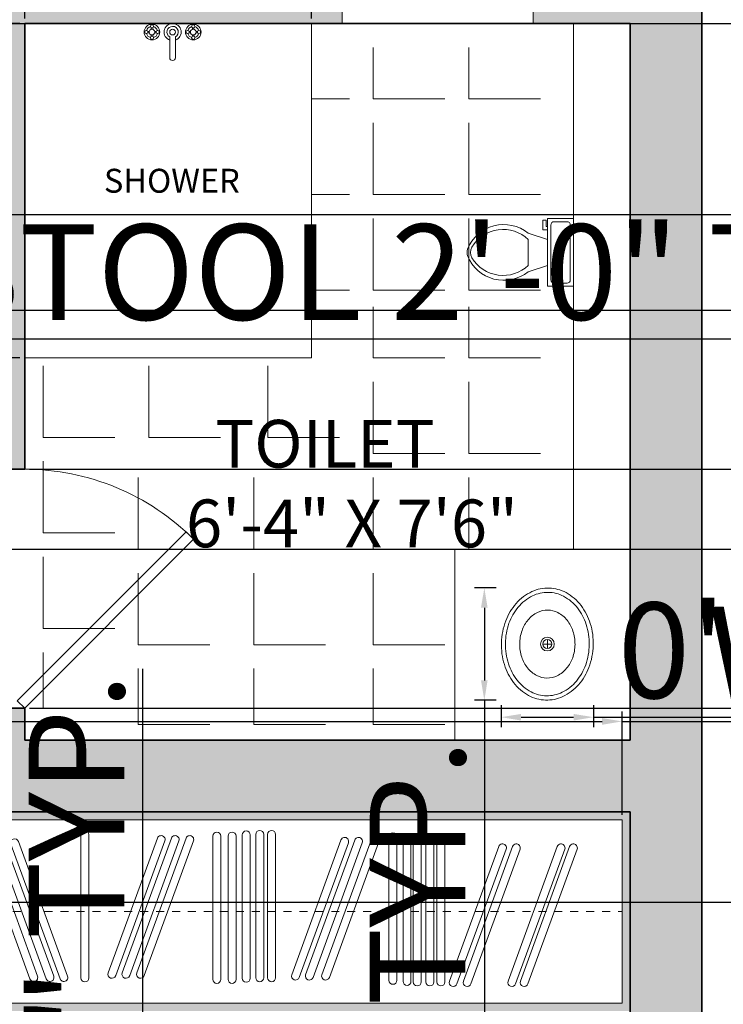
# Model space of a CAD drawing. Units: millimetres. Extents: x 542930 to 543750, y 628093 to 628738.
# Tile 10 of 14: x 543414 to 543502, y 628458 to 628581. Entities that reach past the tile are written whole.
import ezdxf

# ---------------------------------------------------------------- set-up
doc = ezdxf.new("R2010")
doc.units = ezdxf.units.MM
doc.linetypes.add('JIS_02_1.0', pattern=[2, 1, -1])
for name, color, linetype, lineweight in [('A-ANNO-DIMS', 2, 'Continuous', 18), ('A-FLOR-FIXT', 9, 'Continuous', 18), ('A-FURN-MILL', 8, 'Continuous', 18), ('A-FURN-MILL-HIDN', 8, 'JIS_02_1.0', 13), ('A-FURN-PATT', 9, 'Continuous', 13), ('A-WALL', 7, 'Continuous', 35), ('DOORS', 30, 'Continuous', 18), ('WINDOW', 70, 'Continuous', 18)]:
    doc.layers.add(name, color=color, linetype=linetype, lineweight=lineweight)
for name, color, linetype, lineweight, true_color in [('A-ANNO-TEXT', 40, 'Continuous', 18, 0xf8d731), ('A-AREA-IDEN', 40, 'Continuous', 18, 0xf8d731), ('A-FLOR-PATT', 241, 'Continuous', 13, 0xf7abae), ('A-WALL-PATT', 251, 'Continuous', 13, 0x636466)]:
    doc.layers.add(name, color=color, linetype=linetype, lineweight=lineweight, true_color=true_color)
doc.styles.get("Standard").update_dxf_attribs({"font": 'arial.ttf'})
doc.dimstyles.new('ISO-25', dxfattribs={"dimtxt": 12, "dimasz": 2.5, "dimexe": 1.25, "dimexo": 0.625, "dimtad": 1, "dimdec": 0, "dimlunit": 3, "dimtxsty": 'Standard', "dimcen": 2.5, "dimadec": 0, "dimazin": 0, "dimtfac": 1, "dimtdec": 0, "dimtmove": 0, "dimatfit": 3, "dimfxl": 1, "dimarcsym": 0})

# ---------------------------------------------------------------- blocks, each defined once
blk = doc.blocks.new('*U3')
for p, q in [((-40, 0), (-40, -6)), ((0, 0), (0, -6))]:
    blk.add_line(p, q)
blk.add_lwpolyline([(0, 0), (-28.28, 28.28), (-29.52, 27.05), (-1.24, -1.24)], close=True)
blk.add_arc((0, 0), 40, 135, 180)
blk = doc.blocks.new('*U6')
for p, q in [((9.5, -6), (9.5, -2)), ((-10, -8.5), (-8, -8.5)), ((-10, -9.5), (-10, -8.5)), ((-8, -8.5), (-8, -8)), ((-7, -8), (-7, -9.5)), ((-4, -8), (-6, -14)), ((4, -8), (6, -14)), ((-7, -9.5), (-10, -9.5)), ((4, -14), (-4, -14))]:
    blk.add_line(p, q)
blk.add_lwpolyline([(10.5, -8), (10.5, 0), (-10.5, 0), (-10.5, -8)], close=True)
for points in [[(-9.5, -2), (-9.5, -6)], [(8.5, -1), (-8.5, -1)], [(-8.5, -7), (8.5, -7)]]:
    blk.add_lwpolyline(points)
for centre, radius, start, end in [((-8.62, -1.88), 0.884, 81.8699, 188.1301), ((8.62, -1.88), 0.884, 351.8699, 98.1301), ((-8.62, -6.12), 0.884, 171.8699, 278.1301), ((8.62, -6.12), 0.884, 261.8699, 8.1301), ((3.52, -21.58), 12.17, 141.4691, 247.9714), ((4.2, -21.82), 11.33, 136.3677, 238.9468), ((-3.52, -21.58), 12.17, 292.0284, 38.5307), ((-4.2, -21.82), 11.33, 301.053, 43.6321), ((0, -27.88), 4, 245.7318, 294.2682), ((0, -29), 4, 254.8605, 285.1395)]:
    blk.add_arc(centre, radius, start, end)
blk = doc.blocks.new('Sink - Oval top')
for p, q in [((-1, 0), (1, 0)), ((0, 1), (0, -1))]:
    blk.add_line(p, q)
for points in [[(-12.23, 0.39, 0.117634), (-11.46, -3.36, 0.104469), (-8.88, -6.8, 0.090016), (-5.08, -9.07, 0.08192), (-0.32, -10.02, 0.08192), (4.49, -9.38, 0.090016), (8.42, -7.36, 0.104469), (11.22, -4.09, 0.117634), (12.23, -0.39, 0.117634), (11.46, 3.36, 0.104469), (8.88, 6.8, 0.090016), (5.08, 9.07, 0.08192), (0.32, 10.02, 0.08192), (-4.49, 9.38, 0.090016), (-8.42, 7.36, 0.104469), (-11.22, 4.09, 0.117634)], [(-11.29, 0.16, 0.118622), (-10.52, -3.25, 0.104678), (-8.07, -6.36, 0.089562), (-4.54, -8.37, 0.081185), (-0.13, -9.15, 0.081185), (4.3, -8.49, 0.089562), (7.89, -6.58, 0.104678), (10.42, -3.55, 0.118622), (11.29, -0.16, 0.118622), (10.52, 3.25, 0.104678), (8.07, 6.36, 0.089562), (4.54, 8.37, 0.081185), (0.13, 9.15, 0.081185), (-4.3, 8.49, 0.089562), (-7.89, 6.58, 0.104678), (-10.42, 3.55, 0.118622)], [(-7.42, 0.08, 0.118283), (-6.91, -2.17, 0.104607), (-5.29, -4.21, 0.089718), (-2.97, -5.53, 0.081436), (-0.07, -6.04, 0.081436), (2.84, -5.59, 0.089718), (5.2, -4.33, 0.104607), (6.86, -2.32, 0.118283), (7.42, -0.08, 0.118283), (6.91, 2.17, 0.104607), (5.29, 4.21, 0.089718), (2.97, 5.53, 0.081436), (0.07, 6.04, 0.081436), (-2.84, 5.59, 0.089718), (-5.2, 4.33, 0.104607), (-6.86, 2.32, 0.118283)]]:
    blk.add_lwpolyline(points, format="xyb", close=True)
for radius in [1.5, 1]:
    blk.add_circle((0, 0), radius)
blk = doc.blocks.new('Faucet - Bathroom top')
for p, q in [((-4.107, 0.125), (-4.375, 0.125)), ((-3.75, 0.4788), (-3.75, 0.75)), ((-3.5, 0.482), (-3.5, 0.75)), ((-3.1461, 0.125), (-2.875, 0.125)), ((3.143, 0.125), (2.875, 0.125)), ((3.5, 0.4788), (3.5, 0.75)), ((3.75, 0.482), (3.75, 0.75)), ((4.1039, 0.125), (4.375, 0.125)), ((-4.1039, -0.125), (-4.375, -0.125)), ((-3.75, -0.4821), (-3.75, -0.75)), ((-3.5, -0.4789), (-3.5, -0.75)), ((-3.143, -0.125), (-2.875, -0.125)), ((-0.5, -0.8639), (-0.5, -4.5)), ((0.5, -4.5), (0.5, -0.8631)), ((3.1461, -0.125), (2.875, -0.125)), ((3.5, -0.4821), (3.5, -0.75)), ((3.75, -0.4789), (3.75, -0.75)), ((4.107, -0.125), (4.375, -0.125))]:
    blk.add_line(p, q)
for centre, radius in [((-3.625, 0), 1.375), ((-4.625, 0), 0.2795), ((-3.625, 0), 0.5), ((-3.625, 1), 0.2795), ((-2.625, 0), 0.2795), ((0, 0), 0.5), ((3.625, 0), 1.375), ((2.625, 0), 0.2795), ((3.625, 0), 0.5), ((3.625, 1), 0.2795), ((4.625, 0), 0.2795), ((-3.625, -1), 0.2795), ((3.625, -1), 0.2795)]:
    blk.add_circle(centre, radius)
for centre, radius, start, end in [((-3.625, 0), 1, 105.2407, 164.2093), ((-3.625, 0), 1, 16.44125, 74.07887), ((0, 0), 1.5, 289.6514, 250.3603), ((0, 0), 1, 300.3431, 239.7554), ((3.625, 0), 1, 106.12, 164.0884), ((3.625, 0), 1, 16.23422, 73.90469), ((-3.625, 0), 1, 196.2342, 253.9047), ((-3.625, 0), 1, 286.12, 344.0884), ((3.625, 0), 1, 196.4413, 254.0789), ((3.625, 0), 1, 285.2407, 344.2093), ((0, -4.5), 0.5, 180, 0)]:
    blk.add_arc(centre, radius, start, end)
blk = doc.blocks.new('WARDROBE-BED-RAIL')
for p, q in [((0, 23), (0, 0)), ((0, 23), (82.5, 23)), ((82.5, 0), (82.5, 23)), ((14.55, 3.16), (14.55, 21.16)), ((15.55, 3.16), (15.55, 21.16)), ((34.81, 3.12), (34.81, 21.12)), ((35.81, 3.12), (35.81, 21.12)), ((36.51, 3.19), (36.51, 21.19)), ((37.51, 3.19), (37.51, 21.19)), ((38, 3.19), (38, 21.19)), ((39, 3.19), (39, 21.19)), ((8.16, 3.05), (1.98, 19.95)), ((9.1, 3.39), (2.92, 20.3)), ((10.2, 3.05), (4.02, 19.95)), ((11.14, 3.39), (4.96, 20.3)), ((11.95, 3.05), (5.77, 19.95)), ((12.89, 3.39), (6.71, 20.3)), ((17.99, 3.79), (24.17, 20.7)), ((18.92, 3.45), (25.1, 20.36)), ((19.74, 3.79), (25.92, 20.7)), ((20.68, 3.45), (26.86, 20.36)), ((21.57, 3.79), (27.75, 20.7)), ((22.51, 3.45), (28.69, 20.36)), ((31.12, 2.98), (31.12, 20.98)), ((32.12, 2.98), (32.12, 20.98)), ((33.04, 2.98), (33.04, 20.98)), ((34.04, 2.98), (34.04, 20.98)), ((41.02, 3.57), (47.2, 20.48)), ((41.96, 3.23), (48.14, 20.14)), ((42.77, 3.57), (48.95, 20.48)), ((43.71, 3.23), (49.89, 20.14)), ((44.81, 3.57), (50.99, 20.48)), ((45.75, 3.23), (51.93, 20.14)), ((53.23, 2.86), (53.23, 20.86)), ((54.23, 2.86), (54.23, 20.86)), ((55, 2.73), (55, 20.73)), ((56, 2.73), (56, 20.73)), ((56.28, 2.66), (56.28, 20.66)), ((57.28, 2.66), (57.28, 20.66)), ((57.87, 2.66), (57.87, 20.66)), ((58.87, 2.66), (58.87, 20.66)), ((59.26, 2.66), (59.26, 20.66)), ((60.26, 2.66), (60.26, 20.66)), ((60.83, 2.75), (67.01, 19.66)), ((61.77, 2.41), (67.95, 19.31)), ((62.58, 2.75), (68.76, 19.66)), ((63.52, 2.41), (69.7, 19.31)), ((68.19, 2.75), (74.37, 19.66)), ((69.13, 2.41), (75.31, 19.31)), ((69.74, 2.75), (75.92, 19.66)), ((70.68, 2.41), (76.86, 19.31)), ((0, 0), (82.5, 0))]:
    blk.add_line(p, q)
for centre, start, end in [((15.05, 21.16), 0, 180), ((24.63, 20.53), 339.919, 159.919), ((26.39, 20.53), 339.919, 159.919), ((28.22, 20.53), 339.919, 159.919), ((31.62, 20.98), 0, 180), ((33.54, 20.98), 0, 180), ((35.31, 21.12), 0, 180), ((37.01, 21.19), 0, 180), ((38.5, 21.19), 0, 180), ((53.73, 20.86), 0, 180), ((55.5, 20.73), 0, 180), ((56.78, 20.66), 0, 180), ((58.37, 20.66), 0, 180), ((59.76, 20.66), 0, 180), ((2.45, 20.12), 20.081, 200.081), ((4.49, 20.12), 20.081, 200.081), ((6.24, 20.12), 20.081, 200.081), ((47.67, 20.31), 339.919, 159.919), ((49.42, 20.31), 339.919, 159.919), ((51.46, 20.31), 339.919, 159.919), ((67.48, 19.49), 339.919, 159.919), ((69.23, 19.49), 339.919, 159.919), ((74.84, 19.49), 339.919, 159.919), ((76.39, 19.49), 339.919, 159.919), ((18.45, 3.62), 159.919, 339.919), ((20.21, 3.62), 159.919, 339.919), ((22.04, 3.62), 159.919, 339.919), ((8.63, 3.22), 200.081, 20.081), ((10.67, 3.22), 200.081, 20.081), ((12.42, 3.22), 200.081, 20.081), ((15.05, 3.16), 180, 0), ((31.62, 2.98), 180, 0), ((33.54, 2.98), 180, 0), ((35.31, 3.12), 180, 0), ((37.01, 3.19), 180, 0), ((38.5, 3.19), 180, 0), ((41.49, 3.4), 159.919, 339.919), ((43.24, 3.4), 159.919, 339.919), ((45.28, 3.4), 159.919, 339.919), ((53.73, 2.86), 180, 0), ((55.5, 2.73), 180, 0), ((56.78, 2.66), 180, 0), ((58.37, 2.66), 180, 0), ((59.76, 2.66), 180, 0), ((61.3, 2.58), 159.919, 339.919), ((63.05, 2.58), 159.919, 339.919), ((68.66, 2.58), 159.919, 339.919), ((70.21, 2.58), 159.919, 339.919)]:
    blk.add_arc(centre, 0.5, start, end)
blk = doc.blocks.new('SHOWER-ENCLOSURE')
for p, q in [((36, 0), (36, 42)), ((0, 0), (36, 0))]:
    blk.add_line(p, q)
blk = doc.blocks.new('LAVATORY-COUNTER')
for p, q in [((0, 0), (0, 24)), ((0, 24), (22, 24))]:
    blk.add_line(p, q)
blk = doc.blocks.new('*D35')
at = {"layer": 'A-ANNO-DIMS', "color": 0, "lineweight": -2, "transparency": 16777216}
for p, q in [((543473.87, 628509.97), (543471.13, 628509.97)), ((543472.38, 628507.47), (543472.38, 628498.35)), ((543473.87, 628495.85), (543471.13, 628495.85)), ((543472.38, 628495.85), (543472.38, 628364.52))]:
    blk.add_line(p, q, dxfattribs=at)
at = {"layer": 'A-ANNO-DIMS', "color": 0, "transparency": 16777216}
for points in [[(543471.96, 628507.47), (543472.79, 628507.47), (543472.38, 628509.97)], [(543471.96, 628498.35), (543472.79, 628498.35), (543472.38, 628495.85)]]:
    blk.add_solid(points, dxfattribs=at)
at = {"layer": 'Defpoints', "color": 0, "transparency": 16777216}
for p in [(543474.49, 628509.97), (543472.38, 628495.85), (543474.49, 628495.85)]:
    blk.add_point(p, dxfattribs=at)
at = {"layer": 'A-ANNO-DIMS', "color": 0, "transparency": 16777216, "insert": (543465.55, 628428.93), "char_height": 12, "attachment_point": 5, "rotation": 90}
blk.add_mtext('BASIN 1\'-2" TYP.', dxfattribs=at)
blk = doc.blocks.new('*D36')
at = {"layer": 'A-ANNO-DIMS', "color": 0, "lineweight": -2, "transparency": 16777216}
for p, q in [((543474.49, 628495.22), (543474.49, 628492.48)), ((543486.08, 628495.22), (543486.08, 628492.48)), ((543476.99, 628493.73), (543483.58, 628493.73)), ((543486.08, 628493.73), (543600.26, 628493.73))]:
    blk.add_line(p, q, dxfattribs=at)
at = {"layer": 'A-ANNO-DIMS', "color": 0, "transparency": 16777216}
for points in [[(543476.99, 628494.14), (543476.99, 628493.31), (543474.49, 628493.73)], [(543483.58, 628494.14), (543483.58, 628493.31), (543486.08, 628493.73)]]:
    blk.add_solid(points, dxfattribs=at)
at = {"layer": 'Defpoints', "color": 0, "transparency": 16777216}
for p in [(543474.49, 628495.85), (543486.08, 628495.85), (543486.08, 628493.73)]:
    blk.add_point(p, dxfattribs=at)
at = {"layer": 'A-ANNO-DIMS', "color": 0, "transparency": 16777216, "insert": (543544.42, 628500.56), "char_height": 12, "attachment_point": 5}
blk.add_mtext('0\'-11 1/2" TYP.', dxfattribs=at)
blk = doc.blocks.new('*D37')
at = {"layer": 'A-ANNO-DIMS', "color": 0, "lineweight": -2, "transparency": 16777216}
for p, q in [((543337.17, 628423.55), (543337.17, 628436.21)), ((543417.44, 628423.55), (543417.44, 628436.21)), ((543337.17, 628434.96), (543128.93, 628434.96)), ((543414.94, 628434.96), (543339.67, 628434.96))]:
    blk.add_line(p, q, dxfattribs=at)
at = {"layer": 'A-ANNO-DIMS', "color": 0, "transparency": 16777216}
for points in [[(543339.67, 628435.38), (543339.67, 628434.55), (543337.17, 628434.96)], [(543414.94, 628435.38), (543414.94, 628434.55), (543417.44, 628434.96)]]:
    blk.add_solid(points, dxfattribs=at)
at = {"layer": 'Defpoints', "color": 0, "transparency": 16777216}
for p in [(543337.17, 628434.96), (543337.17, 628422.92), (543417.44, 628422.92)]:
    blk.add_point(p, dxfattribs=at)
at = {"layer": 'A-ANNO-DIMS', "color": 0, "transparency": 16777216, "insert": (543231.8, 628442.16), "char_height": 12, "attachment_point": 5}
blk.add_mtext('QUEEN BED 6\'-8 1/2" TYP.', dxfattribs=at)
blk = doc.blocks.new('*D38')
at = {"layer": 'A-ANNO-DIMS', "color": 0, "lineweight": -2, "transparency": 16777216}
for p, q in [((543429.48, 628422.92), (543429.48, 628499.82)), ((543418.07, 628422.92), (543430.73, 628422.92)), ((543429.48, 628365.22), (543429.48, 628420.42)), ((543418.07, 628362.72), (543430.73, 628362.72))]:
    blk.add_line(p, q, dxfattribs=at)
at = {"layer": 'A-ANNO-DIMS', "color": 0, "transparency": 16777216}
for points in [[(543429.07, 628420.42), (543429.9, 628420.42), (543429.48, 628422.92)], [(543429.07, 628365.22), (543429.9, 628365.22), (543429.48, 628362.72)]]:
    blk.add_solid(points, dxfattribs=at)
at = {"layer": 'Defpoints', "color": 0, "transparency": 16777216}
for p in [(543417.44, 628422.92), (543429.48, 628422.92), (543417.44, 628362.72)]:
    blk.add_point(p, dxfattribs=at)
at = {"layer": 'A-ANNO-DIMS', "color": 0, "transparency": 16777216, "insert": (543422.73, 628462.62), "char_height": 12, "attachment_point": 5, "rotation": 90}
blk.add_mtext('5\'-0" TYP.', dxfattribs=at)
blk = doc.blocks.new('*D45')
at = {"layer": 'A-ANNO-DIMS', "color": 0, "lineweight": -2, "transparency": 16777216}
for p, q in [((543407.17, 628481.45), (543407.17, 628494.45)), ((543489.67, 628481.45), (543489.67, 628494.45)), ((543409.67, 628493.2), (543487.17, 628493.2)), ((543489.67, 628493.2), (543749.65, 628493.2))]:
    blk.add_line(p, q, dxfattribs=at)
at = {"layer": 'A-ANNO-DIMS', "color": 0, "transparency": 16777216}
for points in [[(543409.67, 628493.62), (543409.67, 628492.78), (543407.17, 628493.2)], [(543487.17, 628493.62), (543487.17, 628492.78), (543489.67, 628493.2)]]:
    blk.add_solid(points, dxfattribs=at)
at = {"layer": 'Defpoints', "color": 0, "transparency": 16777216}
for p in [(543489.67, 628493.2), (543407.17, 628480.83), (543489.67, 628480.83)]:
    blk.add_point(p, dxfattribs=at)
at = {"layer": 'A-ANNO-DIMS', "color": 0, "transparency": 16777216, "insert": (543620.91, 628500.03), "char_height": 12, "attachment_point": 5}
blk.add_mtext('WARDROBE RAIL 6\'-10 1/2" TYP.', dxfattribs=at)
blk = doc.blocks.new('*D53')
at = {"layer": 'A-ANNO-DIMS', "color": 0, "lineweight": -2, "transparency": 16777216}
for p, q in [((543408.37, 628580.83), (543408.37, 628737.76)), ((543414.04, 628580.83), (543407.12, 628580.83)), ((543408.37, 628541.33), (543408.37, 628578.33)), ((543414.04, 628538.83), (543407.12, 628538.83))]:
    blk.add_line(p, q, dxfattribs=at)
at = {"layer": 'A-ANNO-DIMS', "color": 0, "transparency": 16777216}
for points in [[(543407.95, 628578.33), (543408.78, 628578.33), (543408.37, 628580.83)], [(543407.95, 628541.33), (543408.78, 628541.33), (543408.37, 628538.83)]]:
    blk.add_solid(points, dxfattribs=at)
at = {"layer": 'Defpoints', "color": 0, "transparency": 16777216}
for p in [(543408.37, 628580.83), (543414.67, 628580.83), (543414.67, 628538.83)]:
    blk.add_point(p, dxfattribs=at)
at = {"layer": 'A-ANNO-DIMS', "color": 0, "transparency": 16777216, "insert": (543401.53, 628660.54), "char_height": 12, "attachment_point": 5, "rotation": 90}
blk.add_mtext('SHOWER 3\'-6" TYP.', dxfattribs=at)
blk = doc.blocks.new('*D54')
at = {"layer": 'A-ANNO-DIMS', "color": 0, "lineweight": -2, "transparency": 16777216}
for p, q in [((543414.67, 628581.45), (543414.67, 628588.38)), ((543450.67, 628581.45), (543450.67, 628588.38)), ((543417.17, 628587.13), (543448.17, 628587.13)), ((543450.67, 628587.13), (543527.55, 628587.13))]:
    blk.add_line(p, q, dxfattribs=at)
at = {"layer": 'A-ANNO-DIMS', "color": 0, "transparency": 16777216}
for points in [[(543417.17, 628587.54), (543417.17, 628586.71), (543414.67, 628587.13)], [(543448.17, 628587.54), (543448.17, 628586.71), (543450.67, 628587.13)]]:
    blk.add_solid(points, dxfattribs=at)
at = {"layer": 'Defpoints', "color": 0, "transparency": 16777216}
for p in [(543450.67, 628587.13), (543414.67, 628580.83), (543450.67, 628580.83)]:
    blk.add_point(p, dxfattribs=at)
at = {"layer": 'A-ANNO-DIMS', "color": 0, "transparency": 16777216, "insert": (543490.36, 628593.88), "char_height": 12, "attachment_point": 5}
blk.add_mtext('3\'-0" TYP.', dxfattribs=at)
blk = doc.blocks.new('*D57')
at = {"layer": 'A-ANNO-DIMS', "color": 0, "lineweight": -2, "transparency": 16777216}
for p, q in [((543374.67, 628544.2), (543374.67, 628539.98)), ((543398.67, 628544.2), (543398.67, 628539.98)), ((543377.17, 628541.23), (543396.17, 628541.23)), ((543398.67, 628541.23), (543536.99, 628541.23))]:
    blk.add_line(p, q, dxfattribs=at)
at = {"layer": 'A-ANNO-DIMS', "color": 0, "transparency": 16777216}
for points in [[(543377.17, 628541.64), (543377.17, 628540.81), (543374.67, 628541.23)], [(543396.17, 628541.64), (543396.17, 628540.81), (543398.67, 628541.23)]]:
    blk.add_solid(points, dxfattribs=at)
at = {"layer": 'Defpoints', "color": 0, "transparency": 16777216}
for p in [(543374.67, 628544.83), (543398.67, 628544.83), (543398.67, 628541.23)]:
    blk.add_point(p, dxfattribs=at)
at = {"layer": 'A-ANNO-DIMS', "color": 0, "transparency": 16777216, "insert": (543469.08, 628548.06), "char_height": 12, "attachment_point": 5}
blk.add_mtext('STOOL 2\'-0" TYP.', dxfattribs=at)
blk = doc.blocks.new('*D70')
at = {"layer": 'A-ANNO-DIMS', "color": 0, "lineweight": -2, "transparency": 16777216}
for p, q in [((543325.79, 628580.83), (543537.81, 628580.83)), ((543536.56, 628517.33), (543536.56, 628578.33)), ((543325.79, 628514.83), (543537.81, 628514.83))]:
    blk.add_line(p, q, dxfattribs=at)
at = {"layer": 'A-ANNO-DIMS', "color": 0, "transparency": 16777216}
for points in [[(543536.15, 628578.33), (543536.98, 628578.33), (543536.56, 628580.83)], [(543536.15, 628517.33), (543536.98, 628517.33), (543536.56, 628514.83)]]:
    blk.add_solid(points, dxfattribs=at)
at = {"layer": 'Defpoints', "color": 0, "transparency": 16777216}
for p in [(543325.17, 628580.83), (543536.56, 628580.83), (543325.17, 628514.83)]:
    blk.add_point(p, dxfattribs=at)
at = {"layer": 'A-ANNO-DIMS', "color": 0, "transparency": 16777216, "insert": (543529.81, 628547.83), "char_height": 12, "attachment_point": 5, "rotation": 90}
blk.add_mtext('5\'-6"', dxfattribs=at)
blk = doc.blocks.new('*D72')
at = {"layer": 'A-ANNO-DIMS', "color": 0, "lineweight": -2, "transparency": 16777216}
for p, q in [((543536.56, 628544.83), (543536.56, 628580.68)), ((543282.29, 628544.83), (543537.81, 628544.83)), ((543536.56, 628517.33), (543536.56, 628542.33)), ((543282.29, 628514.83), (543537.81, 628514.83))]:
    blk.add_line(p, q, dxfattribs=at)
at = {"layer": 'A-ANNO-DIMS', "color": 0, "transparency": 16777216}
for points in [[(543536.15, 628542.33), (543536.98, 628542.33), (543536.56, 628544.83)], [(543536.15, 628517.33), (543536.98, 628517.33), (543536.56, 628514.83)]]:
    blk.add_solid(points, dxfattribs=at)
at = {"layer": 'Defpoints', "color": 0, "transparency": 16777216}
for p in [(543281.67, 628544.83), (543536.56, 628544.83), (543281.67, 628514.83)]:
    blk.add_point(p, dxfattribs=at)
at = {"layer": 'A-ANNO-DIMS', "color": 0, "transparency": 16777216, "insert": (543529.81, 628564), "char_height": 12, "attachment_point": 5, "rotation": 90}
blk.add_mtext('2\'-6"', dxfattribs=at)
blk = doc.blocks.new('*D77')
at = {"layer": 'A-ANNO-DIMS', "color": 0, "lineweight": -2, "transparency": 16777216}
for p, q in [((543536.56, 628524.86), (543536.56, 628560.72)), ((543415.29, 628524.86), (543537.81, 628524.86)), ((543536.56, 628497.36), (543536.56, 628522.36)), ((543415.29, 628494.86), (543537.81, 628494.86))]:
    blk.add_line(p, q, dxfattribs=at)
at = {"layer": 'A-ANNO-DIMS', "color": 0, "transparency": 16777216}
for points in [[(543536.15, 628522.36), (543536.98, 628522.36), (543536.56, 628524.86)], [(543536.15, 628497.36), (543536.98, 628497.36), (543536.56, 628494.86)]]:
    blk.add_solid(points, dxfattribs=at)
at = {"layer": 'Defpoints', "color": 0, "transparency": 16777216}
for p in [(543414.67, 628524.86), (543536.56, 628524.86), (543414.67, 628494.86)]:
    blk.add_point(p, dxfattribs=at)
at = {"layer": 'A-ANNO-DIMS', "color": 0, "transparency": 16777216, "insert": (543529.81, 628544.04), "char_height": 12, "attachment_point": 5, "rotation": 90}
blk.add_mtext('2\'-6"', dxfattribs=at)
blk = doc.blocks.new('*D80')
at = {"layer": 'A-ANNO-DIMS', "color": 0, "lineweight": -2, "transparency": 16777216}
for p, q in [((543228.79, 628470.52), (543537.81, 628470.52)), ((543536.56, 628437.09), (543536.56, 628468.02)), ((543228.79, 628434.59), (543537.81, 628434.59))]:
    blk.add_line(p, q, dxfattribs=at)
at = {"layer": 'A-ANNO-DIMS', "color": 0, "transparency": 16777216}
for points in [[(543536.15, 628468.02), (543536.98, 628468.02), (543536.56, 628470.52)], [(543536.15, 628437.09), (543536.98, 628437.09), (543536.56, 628434.59)]]:
    blk.add_solid(points, dxfattribs=at)
at = {"layer": 'Defpoints', "color": 0, "transparency": 16777216}
for p in [(543228.16, 628470.52), (543536.56, 628470.52), (543228.16, 628434.59)]:
    blk.add_point(p, dxfattribs=at)
at = {"layer": 'A-ANNO-DIMS', "color": 0, "transparency": 16777216, "insert": (543529.81, 628452.55), "char_height": 12, "attachment_point": 5, "rotation": 90}
blk.add_mtext('3\'-0"', dxfattribs=at)
blk = doc.blocks.new('*D83')
at = {"layer": 'A-ANNO-DIMS', "color": 0, "lineweight": -2, "transparency": 16777216}
for p, q in [((543536.56, 628580.83), (543536.56, 628616.68)), ((543410.79, 628580.83), (543537.81, 628580.83)), ((543536.56, 628559.33), (543536.56, 628578.33)), ((543410.79, 628556.83), (543537.81, 628556.83))]:
    blk.add_line(p, q, dxfattribs=at)
at = {"layer": 'A-ANNO-DIMS', "color": 0, "transparency": 16777216}
for points in [[(543536.15, 628578.33), (543536.98, 628578.33), (543536.56, 628580.83)], [(543536.15, 628559.33), (543536.98, 628559.33), (543536.56, 628556.83)]]:
    blk.add_solid(points, dxfattribs=at)
at = {"layer": 'Defpoints', "color": 0, "transparency": 16777216}
for p in [(543410.17, 628580.83), (543536.56, 628580.83), (543410.17, 628556.83)]:
    blk.add_point(p, dxfattribs=at)
at = {"layer": 'A-ANNO-DIMS', "color": 0, "transparency": 16777216, "insert": (543529.81, 628600), "char_height": 12, "attachment_point": 5, "rotation": 90}
blk.add_mtext('2\'-0"', dxfattribs=at)
blk = doc.blocks.new('*D84')
at = {"layer": 'A-ANNO-DIMS', "color": 0, "lineweight": -2, "transparency": 16777216}
for p, q in [((543386.67, 628556.2), (543386.67, 628103.84)), ((543370.17, 628490.2), (543370.17, 628103.84)), ((543372.67, 628105.09), (543384.17, 628105.09)), ((543386.67, 628105.09), (543449.15, 628105.09))]:
    blk.add_line(p, q, dxfattribs=at)
at = {"layer": 'A-ANNO-DIMS', "color": 0, "transparency": 16777216}
for points in [[(543372.67, 628105.5), (543372.67, 628104.67), (543370.17, 628105.09)], [(543384.17, 628105.5), (543384.17, 628104.67), (543386.67, 628105.09)]]:
    blk.add_solid(points, dxfattribs=at)
at = {"layer": 'Defpoints', "color": 0, "transparency": 16777216}
for p in [(543386.67, 628556.83), (543370.17, 628490.83), (543386.67, 628105.09)]:
    blk.add_point(p, dxfattribs=at)
at = {"layer": 'A-ANNO-DIMS', "color": 0, "transparency": 16777216, "insert": (543419.16, 628111.92), "char_height": 12, "attachment_point": 5}
blk.add_mtext('1\'-4 1/2"', dxfattribs=at)

msp = doc.modelspace()

# ---------------------------------------------------------------- hatches: boundary and pattern name
at = {"layer": 'A-FURN-PATT'}
h = msp.add_hatch(color=256, dxfattribs=at)
h.dxf.hatch_style = 1
h.paths.add_polyline_path([(543490.67, 628481.83), (543406.17, 628481.83), (543406.17, 628456.83), (543490.67, 628456.83)])
h.paths.add_polyline_path([(543407.17, 628480.83), (543489.67, 628480.83), (543489.67, 628457.83), (543407.17, 628457.83)], flags=16)
h.paths.add_polyline_path([(543409.15, 628477.78, -1), (543410.09, 628478.12), (543413.3, 628469.33), (543414.27, 628469.33), (543411.18, 628477.78, -1), (543412.12, 628478.12), (543415.34, 628469.33), (543416.03, 628469.33), (543412.94, 628477.78, -1), (543413.88, 628478.12), (543417.09, 628469.33), (543421.72, 628469.33), (543421.72, 628478.99, -1), (543422.72, 628478.99), (543422.72, 628469.33), (543427.97, 628469.33), (543431.33, 628478.53, -1), (543432.27, 628478.18), (543429.03, 628469.33), (543429.72, 628469.33), (543433.09, 628478.53, -1), (543434.03, 628478.18), (543430.79, 628469.33), (543431.55, 628469.33), (543434.91, 628478.53, -1), (543435.85, 628478.18), (543432.61, 628469.33), (543438.29, 628469.33), (543438.29, 628478.81, -1), (543439.29, 628478.81), (543439.29, 628469.33), (543440.2, 628469.33), (543440.2, 628478.81, -1), (543441.2, 628478.81), (543441.2, 628469.33), (543441.98, 628469.33), (543441.98, 628478.95, -1), (543442.98, 628478.95), (543442.98, 628469.33), (543443.68, 628469.33), (543443.68, 628479.02, -1), (543444.68, 628479.02), (543444.68, 628469.33), (543445.17, 628469.33), (543445.17, 628479.02, -1), (543446.17, 628479.02), (543446.17, 628469.33), (543451.08, 628469.33), (543454.37, 628478.31, -1), (543455.31, 628477.96), (543452.15, 628469.33), (543452.84, 628469.33), (543456.12, 628478.31, -1), (543457.06, 628477.96), (543453.9, 628469.33), (543454.88, 628469.33), (543458.16, 628478.31, -1), (543459.1, 628477.96), (543455.94, 628469.33), (543460.39, 628469.33), (543460.39, 628478.68, -1), (543461.39, 628478.68), (543461.39, 628469.33), (543462.17, 628469.33), (543462.17, 628478.56, -1), (543463.17, 628478.56), (543463.17, 628469.33), (543463.45, 628469.33), (543463.45, 628478.49, -1), (543464.45, 628478.49), (543464.45, 628469.33), (543465.03, 628469.33), (543465.03, 628478.49, -1), (543466.03, 628478.49), (543466.03, 628469.33), (543466.43, 628469.33), (543466.43, 628478.49, -1), (543467.43, 628478.49), (543467.43, 628469.33), (543471.19, 628469.33), (543474.18, 628477.48, -1), (543475.11, 628477.14), (543472.26, 628469.33), (543472.95, 628469.33), (543475.93, 628477.48, -1), (543476.87, 628477.14), (543474.01, 628469.33), (543478.55, 628469.33), (543481.53, 628477.48, -1), (543482.47, 628477.14), (543479.62, 628469.33), (543480.1, 628469.33), (543483.09, 628477.48, -1), (543484.02, 628477.14), (543477.84, 628460.23, -1), (543476.91, 628460.58), (543480.1, 628469.33), (543479.62, 628469.33), (543476.29, 628460.23, -1), (543475.35, 628460.58), (543478.55, 628469.33), (543474.01, 628469.33), (543470.69, 628460.23, -1), (543469.75, 628460.58), (543472.95, 628469.33), (543472.26, 628469.33), (543468.93, 628460.23, -1), (543468, 628460.58), (543471.19, 628469.33), (543467.43, 628469.33), (543467.43, 628460.49, -1), (543466.43, 628460.49), (543466.43, 628469.33), (543466.03, 628469.33), (543466.03, 628460.49, -1), (543465.03, 628460.49), (543465.03, 628469.33), (543464.45, 628469.33), (543464.45, 628460.49, -1), (543463.45, 628460.49), (543463.45, 628469.33), (543463.17, 628469.33), (543463.17, 628460.56, -1), (543462.17, 628460.56), (543462.17, 628469.33), (543461.39, 628469.33), (543461.39, 628460.68, -1), (543460.39, 628460.68), (543460.39, 628469.33), (543455.94, 628469.33), (543452.92, 628461.06, -1), (543451.98, 628461.4), (543454.88, 628469.33), (543453.9, 628469.33), (543450.88, 628461.06, -1), (543449.94, 628461.4), (543452.84, 628469.33), (543452.15, 628469.33), (543449.13, 628461.06, -1), (543448.19, 628461.4), (543451.08, 628469.33), (543446.17, 628469.33), (543446.17, 628461.02, -1), (543445.17, 628461.02), (543445.17, 628469.33), (543444.68, 628469.33), (543444.68, 628461.02, -1), (543443.68, 628461.02), (543443.68, 628469.33), (543442.98, 628469.33), (543442.98, 628460.95, -1), (543441.98, 628460.95), (543441.98, 628469.33), (543441.2, 628469.33), (543441.2, 628460.81, -1), (543440.2, 628460.81), (543440.2, 628469.33), (543439.29, 628469.33), (543439.29, 628460.81, -1), (543438.29, 628460.81), (543438.29, 628469.33), (543432.61, 628469.33), (543429.67, 628461.28, -1), (543428.73, 628461.62), (543431.55, 628469.33), (543430.79, 628469.33), (543427.85, 628461.28, -1), (543426.91, 628461.62), (543429.72, 628469.33), (543429.03, 628469.33), (543426.09, 628461.28, -1), (543425.15, 628461.62), (543427.97, 628469.33), (543422.72, 628469.33), (543422.72, 628460.99, -1), (543421.72, 628460.99), (543421.72, 628469.33), (543417.09, 628469.33), (543420.06, 628461.22, -1), (543419.12, 628460.87), (543416.03, 628469.33), (543415.34, 628469.33), (543418.3, 628461.22, -1), (543417.36, 628460.87), (543414.27, 628469.33), (543413.3, 628469.33), (543416.27, 628461.22, -1), (543415.33, 628460.87)], flags=0)
at = {"layer": 'A-WALL-PATT'}
h = msp.add_hatch(color=256, dxfattribs=at)
h.dxf.hatch_style = 1
h.paths.add_polyline_path([(543454.53, 628589.83), (543271.67, 628589.83), (543271.67, 628580.83), (543325.17, 628580.83), (543325.17, 628475.36), (543334.17, 628475.36), (543334.17, 628481.83), (543370.17, 628481.83), (543370.17, 628490.83), (543334.17, 628490.83), (543334.17, 628580.83), (543410.17, 628580.83), (543410.17, 628524.86), (543414.67, 628524.86), (543414.67, 628580.83), (543454.53, 628580.83)])
h = msp.add_hatch(color=256, dxfattribs=at)
h.dxf.hatch_style = 1
h.paths.add_polyline_path([(543499.67, 628589.83), (543478.53, 628589.83), (543478.53, 628580.83), (543490.67, 628580.83), (543490.67, 628490.83), (543414.67, 628490.83), (543414.67, 628494.86), (543410.17, 628494.86), (543410.17, 628490.83), (543406.17, 628490.83), (543406.17, 628481.83), (543490.67, 628481.83), (543490.67, 628340.3), (543499.67, 628340.3)])

# ---------------------------------------------------------------- linework, layer by layer
at = {"layer": 'A-FLOR-FIXT'}
msp.add_line((543483.57, 628514.83), (543483.57, 628580.83), dxfattribs=at)
at = {"layer": 'A-FLOR-PATT'}
for p, q in [((543458.43, 628577.8), (543458.43, 628571.36)), ((543470.43, 628577.8), (543470.43, 628571.36)), ((543450.67, 628571.36), (543455.43, 628571.36)), ((543458.43, 628571.36), (543467.43, 628571.36)), ((543470.43, 628571.36), (543479.43, 628571.36)), ((543458.43, 628568.36), (543458.43, 628559.36)), ((543470.43, 628568.36), (543470.43, 628559.36)), ((543450.67, 628559.36), (543455.43, 628559.36)), ((543458.43, 628559.36), (543467.43, 628559.36)), ((543470.43, 628559.36), (543479.43, 628559.36)), ((543458.43, 628556.36), (543458.43, 628547.36)), ((543470.43, 628556.36), (543470.43, 628547.36)), ((543450.67, 628547.36), (543455.43, 628547.36)), ((543458.43, 628547.36), (543467.43, 628547.36)), ((543470.43, 628547.36), (543479.43, 628547.36)), ((543458.43, 628545.27), (543458.43, 628538.83)), ((543470.43, 628545.27), (543470.43, 628538.83)), ((543458.43, 628538.83), (543467.43, 628538.83)), ((543470.43, 628538.83), (543479.43, 628538.83)), ((543416.99, 628537.86), (543416.99, 628528.86)), ((543430.25, 628537.86), (543430.25, 628528.86)), ((543445.18, 628537.86), (543445.18, 628528.86)), ((543458.43, 628535.83), (543458.43, 628526.83)), ((543470.43, 628535.83), (543470.43, 628526.83)), ((543416.99, 628528.86), (543425.99, 628528.86)), ((543430.25, 628528.86), (543439.25, 628528.86)), ((543445.18, 628528.86), (543454.18, 628528.86)), ((543458.43, 628526.83), (543467.43, 628526.83)), ((543470.43, 628526.83), (543479.43, 628526.83)), ((543416.99, 628525.86), (543416.99, 628516.86)), ((543428.93, 628523.83), (543428.93, 628514.83)), ((543443.42, 628523.83), (543443.42, 628514.83)), ((543458.43, 628523.83), (543458.43, 628514.83)), ((543470.43, 628523.83), (543470.43, 628514.83)), ((543458.43, 628521.27), (543458.43, 628514.83)), ((543416.99, 628516.86), (543425.99, 628516.86)), ((543428.93, 628514.83), (543437.93, 628514.83)), ((543443.42, 628514.83), (543452.42, 628514.83)), ((543458.43, 628514.83), (543467.43, 628514.83)), ((543416.99, 628513.86), (543416.99, 628504.86)), ((543428.93, 628511.83), (543428.93, 628502.83)), ((543443.42, 628511.83), (543443.42, 628502.83)), ((543458.43, 628511.83), (543458.43, 628502.83)), ((543416.99, 628504.86), (543425.99, 628504.86)), ((543428.93, 628502.83), (543437.93, 628502.83)), ((543443.42, 628502.83), (543452.42, 628502.83)), ((543458.43, 628502.83), (543467.43, 628502.83)), ((543416.99, 628501.86), (543416.99, 628494.86)), ((543428.93, 628499.83), (543428.93, 628492.83)), ((543443.42, 628499.83), (543443.42, 628492.83)), ((543458.43, 628499.83), (543458.43, 628492.83)), ((543416.99, 628494.86), (543425.99, 628494.86)), ((543428.93, 628492.83), (543437.93, 628492.83)), ((543443.42, 628492.83), (543452.42, 628492.83)), ((543458.43, 628492.83), (543467.43, 628492.83))]:
    msp.add_line(p, q, dxfattribs=at)
at = {"layer": 'A-FURN-MILL-HIDN'}
msp.add_line((543407.17, 628469.33), (543489.67, 628469.33), dxfattribs=at)
at = {"layer": 'A-WALL'}
for p, q in [((543499.67, 628589.83), (543499.67, 628253.83)), ((543414.67, 628524.86), (543414.67, 628580.83)), ((543414.67, 628580.83), (543490.67, 628580.83)), ((543490.67, 628580.83), (543490.67, 628490.83)), ((543410.17, 628524.86), (543414.67, 628524.86)), ((543410.17, 628494.86), (543414.67, 628494.86)), ((543414.67, 628490.83), (543414.67, 628494.86)), ((543490.67, 628490.83), (543414.67, 628490.83)), ((543490.67, 628481.83), (543406.17, 628481.83)), ((543490.67, 628481.83), (543490.67, 628262.83))]:
    msp.add_line(p, q, dxfattribs=at)
at = {"layer": 'WINDOW'}
for p, q in [((543454.53, 628589.83), (543454.53, 628580.83)), ((543478.53, 628589.83), (543478.53, 628580.83))]:
    msp.add_line(p, q, dxfattribs=at)

# ---------------------------------------------------------------- block references
at = {"layer": 'A-FLOR-FIXT'}
for name, p in [('SHOWER-ENCLOSURE', (543414.67, 628538.83)), ('LAVATORY-COUNTER', (543468.67, 628490.83))]:
    msp.add_blockref(name, p, dxfattribs=at)
at = {"layer": 'A-FLOR-FIXT', "xscale": 0.7146915789431332, "yscale": 0.7146915789431332, "zscale": 0.7146915789431332}
msp.add_blockref('Faucet - Bathroom top', (543433.24, 628579.75), dxfattribs=at)
at = {"layer": 'A-FLOR-FIXT', "rotation": 270}
for name, p, xscale, yscale, zscale in [('*U6', (543483.57, 628552.08), 0.4049257278699833, 0.4049257278699833, 0.4049257278699833), ('Sink - Oval top', (543480.29, 628502.91), 0.5752271451798996, 0.5752271451798996, 0.5752271451798996)]:
    msp.add_blockref(name, p, dxfattribs=dict(at, xscale=xscale, yscale=yscale, zscale=zscale))
at = {"layer": 'A-FURN-MILL'}
msp.add_blockref('WARDROBE-BED-RAIL', (543407.17, 628457.83), dxfattribs=at)
at = {"layer": 'DOORS', "xscale": 0.75, "yscale": 0.75, "zscale": 0.75, "rotation": 270}
msp.add_blockref('*U3', (543414.67, 628494.86), dxfattribs=at)

# ---------------------------------------------------------------- texts
at = {"layer": 'A-ANNO-TEXT', "insert": (543422.78, 628562.58), "char_height": 3, "attachment_point": 1}
msp.add_mtext_dynamic_manual_height_columns('  SHOWER', width=44.748, gutter_width=12.5, heights=[0], dxfattribs=at)
at = {"layer": 'A-AREA-IDEN', "insert": (543434.92, 628531.06), "char_height": 6, "attachment_point": 1}
msp.add_mtext_dynamic_manual_height_columns('  TOILET\\P6\'-4" X 7\'6"', width=44.748, gutter_width=12.5, heights=[0], dxfattribs=at)

# ---------------------------------------------------------------- dimensions: what is measured, and where the dimension line sits
at = {"layer": 'A-ANNO-DIMS'}
for base, p1, p2, angle, text, picture, middle in [((543408.37, 628580.83), (543414.67, 628538.83), (543414.67, 628580.83), 90, 'SHOWER <> TYP.', '*D53', (543401.53, 628660.54)), ((543472.38, 628495.85), (543474.49, 628509.97), (543474.49, 628495.85), 270, 'BASIN <> TYP.', '*D35', (543465.55, 628428.93)), ((543429.48, 628422.92), (543417.44, 628362.72), (543417.44, 628422.92), 90, '<> TYP.', '*D38', (543422.73, 628462.62)), ((543337.17, 628434.96), (543417.44, 628422.92), (543337.17, 628422.92), 180, 'QUEEN BED <> TYP.', '*D37', (543231.8, 628442.16))]:
    dim = msp.add_linear_dim(base=base, p1=p1, p2=p2, angle=angle, text=text, dimstyle='ISO-25', override={"dimdec": 1, "dimlfac": 1, "dimrnd": 0, "dimzin": 1, "dimdsep": 46, "dimlunit": 4, "dimfrac": 2}, dxfattribs=at)
    dim.commit()
    dim.dimension.update_dxf_attribs({"geometry": picture, "text_midpoint": middle})
for base, p1, p2, picture, middle in [((543536.56, 628580.83), (543410.17, 628556.83), (543410.17, 628580.83), '*D83', (543529.81, 628600)), ((543536.56, 628544.83), (543281.67, 628514.83), (543281.67, 628544.83), '*D72', (543529.81, 628564)), ((543536.56, 628580.83), (543325.17, 628514.83), (543325.17, 628580.83), '*D70', (543529.81, 628547.83)), ((543536.56, 628524.86), (543414.67, 628494.86), (543414.67, 628524.86), '*D77', (543529.81, 628544.04)), ((543536.56, 628470.52), (543228.16, 628434.59), (543228.16, 628470.52), '*D80', (543529.81, 628452.55))]:
    dim = msp.add_linear_dim(base=base, p1=p1, p2=p2, angle=90, dimstyle='ISO-25', override={"dimdec": 1, "dimlfac": 1, "dimrnd": 0, "dimzin": 1, "dimdsep": 46, "dimlunit": 4, "dimfrac": 2}, dxfattribs=at)
    dim.commit()
    dim.dimension.update_dxf_attribs({"geometry": picture, "text_midpoint": middle})
for base, p1, p2, text, picture, middle in [((543450.67, 628587.13), (543414.67, 628580.83), (543450.67, 628580.83), '<> TYP.', '*D54', (543490.36, 628593.88)), ((543398.67, 628541.23), (543374.67, 628544.83), (543398.67, 628544.83), 'STOOL <> TYP.', '*D57', (543469.08, 628548.06)), ((543489.67, 628493.2), (543407.17, 628480.83), (543489.67, 628480.83), 'WARDROBE RAIL <> TYP.', '*D45', (543620.91, 628500.03)), ((543486.08, 628493.73), (543474.49, 628495.85), (543486.08, 628495.85), '<> TYP.', '*D36', (543544.42, 628500.56))]:
    dim = msp.add_linear_dim(base=base, p1=p1, p2=p2, text=text, dimstyle='ISO-25', override={"dimdec": 1, "dimlfac": 1, "dimrnd": 0, "dimzin": 1, "dimdsep": 46, "dimlunit": 4, "dimfrac": 2}, dxfattribs=at)
    dim.commit()
    dim.dimension.update_dxf_attribs({"geometry": picture, "text_midpoint": middle})
dim = msp.add_linear_dim(base=(543386.67, 628105.09), p1=(543370.17, 628490.83), p2=(543386.67, 628556.83), dimstyle='ISO-25', override={"dimdec": 1, "dimlfac": 1, "dimrnd": 0, "dimzin": 1, "dimdsep": 46, "dimlunit": 4, "dimfrac": 2}, dxfattribs=at)
dim.commit()
dim.dimension.update_dxf_attribs({"geometry": '*D84', "text_midpoint": (543419.16, 628111.92)})

doc.saveas('drawing.dxf')
